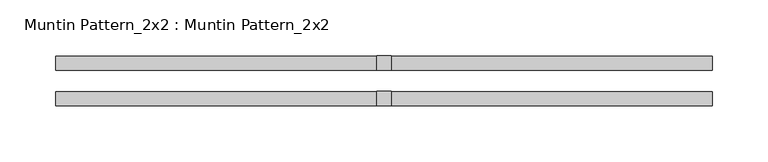
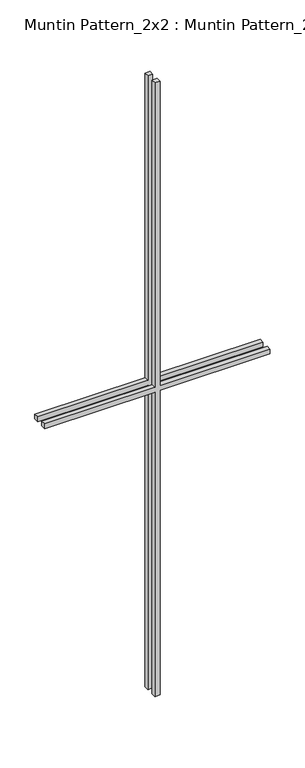
"""IFC4 building model written with IfcOpenShell, lengths in millimetres: proxy geometry, Muntin Pattern_2x2 : Muntin Pattern_2x2."""

from ifc_helpers import new_model, si_unit, frame, origin, place, context, project, spatial, polyline, outline, extrude, source, transform, mapped, element, save


def muntin_pattern_2x2_muntin_pattern_2x2_bff912c5(model_context):
    return source(origin(), model_context, "Body", "SweptSolid", [
        extrude(outline(polyline([(850.9, -6.35), (850.9, -293.6875), (838.2, -293.6875), (838.2, -6.35), (0.0, -6.35), (0.0, 6.35), (838.2, 6.35), (838.2, 293.6875), (850.9, 293.6875), (850.9, 6.35), (1689.1, 6.35), (1689.1, -6.35), (850.9, -6.35)])), frame((0.0, 9.525, 0.0), z_axis=(0.0, 1.0, 0.0), x_axis=(0.0, 0.0, 1.0)), (0.0, 0.0, 1.0), 12.7),
        extrude(outline(polyline([(850.9, -6.35), (850.9, -293.6875), (838.2, -293.6875), (838.2, -6.35), (0.0, -6.35), (0.0, 6.35), (838.2, 6.35), (838.2, 293.6875), (850.9, 293.6875), (850.9, 6.35), (1689.1, 6.35), (1689.1, -6.35), (850.9, -6.35)])), frame((0.0, -22.225, 0.0), z_axis=(0.0, 1.0, 0.0), x_axis=(0.0, 0.0, 1.0)), (0.0, 0.0, 1.0), 12.7),
    ])


if __name__ == "__main__":
    model = new_model("IFC4")
    model_context = context("Model", 3, world=origin())
    ifc_project = project(units=[si_unit("LENGTHUNIT", "METRE", prefix="MILLI")], contexts=[model_context])
    site = spatial("IfcSite", under=ifc_project)
    building = spatial("IfcBuilding", under=site)
    placement = place(None, origin())
    muntin_pattern_2x2_muntin_pattern_2x2_shape = muntin_pattern_2x2_muntin_pattern_2x2_bff912c5(model_context)
    element("IfcBuildingElementProxy", 1, Name="Muntin Pattern_2x2 : Muntin Pattern_2x2", ObjectType="Muntin Pattern_2x2 : Muntin Pattern_2x2", at=placement, inside=building, context=model_context, shape_type="MappedRepresentation", body=[
        mapped(muntin_pattern_2x2_muntin_pattern_2x2_shape, transform((0.0, 0.0, 0.0), x_axis=(1.0, 0.0, 0.0), y_axis=(0.0, 1.0, 0.0), z_axis=(0.0, 0.0, 1.0))),
    ])
    save(model, "model.ifc")

# Revit data of these elements
# Type "Muntin Pattern_2x2 : Muntin Pattern_2x2"
#   Width [instance default] = 4' - 0"
#   Thickness = 0' - 0 1/2"
#   Height [instance default] = 4' - 0"
#   Distance = 0' - 0 3/4"
#   Interior Material [instance default] = none
#   Exterior Material [instance default] = none
#   Default Elevation = 0
# Element 1 (IfcBuildingElementProxy, "Muntin Pattern_2x2 : Muntin Pattern_2x2")
#   Width = 1' - 11 1/8"
#   Height = 5' - 6 1/2"
#   Interior Material = Wood - Stained
#   Exterior Material = Clad - White
#   Materials on its faces: "Clad - White", "Wood - Stained"
# Materials
#   "Clad - White": class "Wood", colour RGB 242 242 238, transparency 0, Cost = 0
#   "Wood - Stained": class "Wood", colour RGB 224 178 126, transparency 0, Cost = 0
